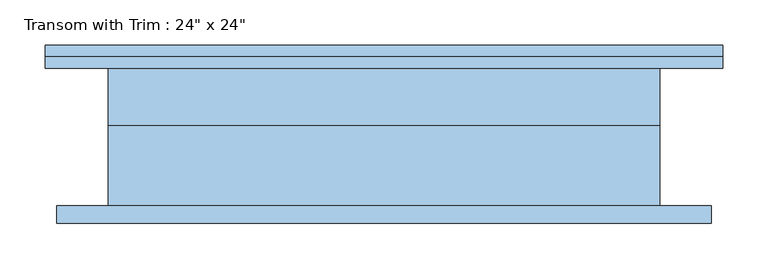
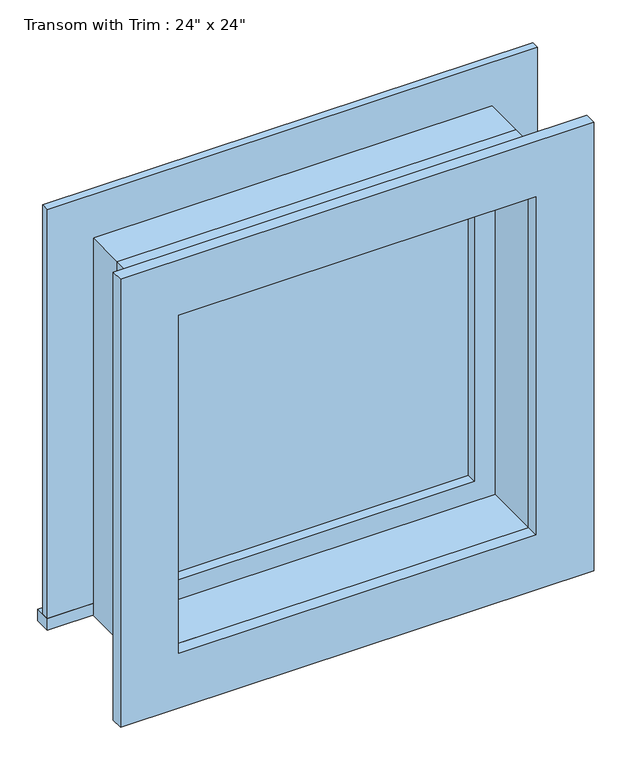
"""IFC4 building model written with IfcOpenShell, lengths in millimetres: window geometry."""

from ifc_helpers import new_model, si_unit, frame, origin, place, context, project, spatial, polyline, outline, extrude, source, transform, mapped, element, save


def window_3d781103(model_context):
    return source(origin(), model_context, "Body", "SweptSolid", [
        extrude(outline(polyline([(-412.75, 101.6), (336.55, 101.6), (336.55, 76.2), (-412.75, 76.2), (-412.75, 101.6)])), frame((0.0, 0.0, 2159.0), z_axis=(0.0, 0.0, 1.0), x_axis=(1.0, 0.0, 0.0)), (0.0, 0.0, 1.0), 19.05),
        extrude(outline(polyline([(2749.55, -323.85), (2749.55, 247.65), (2178.05, 247.65), (2178.05, 336.55), (2838.45, 336.55), (2838.45, -412.75), (2178.05, -412.75), (2178.05, -323.85), (2749.55, -323.85)])), frame((0.0, 76.2, 0.0), z_axis=(0.0, 1.0, 0.0), x_axis=(0.0, 0.0, 1.0)), (0.0, 0.0, 1.0), 12.7),
        extrude(outline(polyline([(2825.75, 323.85), (2825.75, -400.05), (2101.85, -400.05), (2101.85, 323.85), (2825.75, 323.85)]), holes=[polyline([(2736.85, 234.95), (2190.75, 234.95), (2190.75, -311.15), (2736.85, -311.15), (2736.85, 234.95)])]), frame((0.0, -95.25, 0.0), z_axis=(0.0, 1.0, 0.0), x_axis=(0.0, 0.0, 1.0)), (0.0, 0.0, 1.0), 19.05),
        extrude(outline(polyline([(203.2, 28.575), (-279.4, 28.575), (-279.4, 41.275), (203.2, 41.275), (203.2, 28.575)])), frame((0.0, 0.0, 2222.5), z_axis=(0.0, 0.0, 1.0), x_axis=(1.0, 0.0, 0.0)), (0.0, 0.0, 1.0), 482.6),
        extrude(outline(polyline([(2749.55, -323.85), (2178.05, -323.85), (2178.05, 247.65), (2749.55, 247.65), (2749.55, -323.85)]), holes=[polyline([(2705.1, -279.4), (2705.1, 203.2), (2222.5, 203.2), (2222.5, -279.4), (2705.1, -279.4)])]), frame((0.0, 12.7, 0.0), z_axis=(0.0, 1.0, 0.0), x_axis=(0.0, 0.0, 1.0)), (0.0, 0.0, 1.0), 44.45),
        extrude(outline(polyline([(2768.6, -342.9), (2159.0, -342.9), (2159.0, 266.7), (2768.6, 266.7), (2768.6, -342.9)]), holes=[polyline([(2736.85, -311.15), (2736.85, 234.95), (2190.75, 234.95), (2190.75, -311.15), (2736.85, -311.15)])]), frame((0.0, -76.2, 0.0), z_axis=(0.0, 1.0, 0.0), x_axis=(0.0, 0.0, 1.0)), (0.0, 0.0, 1.0), 88.9),
        extrude(outline(polyline([(2768.6, 266.7), (2768.6, -342.9), (2159.0, -342.9), (2159.0, 266.7), (2768.6, 266.7)]), holes=[polyline([(2749.55, 247.65), (2178.05, 247.65), (2178.05, -323.85), (2749.55, -323.85), (2749.55, 247.65)])]), frame((0.0, 12.7, 0.0), z_axis=(0.0, 1.0, 0.0), x_axis=(0.0, 0.0, 1.0)), (0.0, 0.0, 1.0), 63.5),
    ])


if __name__ == "__main__":
    model = new_model("IFC4")
    model_context = context("Model", 3, world=origin())
    ifc_project = project(units=[si_unit("LENGTHUNIT", "METRE", prefix="MILLI")], contexts=[model_context])
    site = spatial("IfcSite", under=ifc_project)
    building = spatial("IfcBuilding", under=site)
    placement = place(None, origin())
    window_shape = window_3d781103(model_context)
    element("IfcWindow", 1, ObjectType="Transom with Trim : 24\" x 24\"", at=placement, inside=building, context=model_context, shape_type="MappedRepresentation", body=[
        mapped(window_shape, transform((0.0, 0.0, 0.0), x_axis=(1.0, 0.0, 0.0), y_axis=(0.0, 1.0, 0.0), z_axis=(0.0, 0.0, 1.0))),
    ])
    save(model, "model.ifc")

# Revit data of these elements
# Type "Transom with Trim : 24\" x 24\""
#   Type Mark = "19"
#   Construction Type Id = "GSP4R"
#   Assembly Code = "B2020100"
#   Analytic Construction = "1/8 in Pilkington single glazing"
#   Visual Light Transmittance = 0.9
#   Solar Heat Gain Coefficient = 0.78
#   Heat Transfer Coefficient (U) = 0.6496 BTU/(h·ft²·°F)
#   Height = 2' - 0"
#   Default Sill Height = 7' - 1"
#   Trim Projection - Ext. = 0' - 0 1/2"
#   Trim Projection - Int. = 0' - 0 3/4"
#   Trim Width - Exterior = 0' - 3 1/2"
#   Trim Width - Interior = 0' - 3 1/2"
#   Width = 2' - 0"
#   Window Inset = 0' - 0 3/4"
#   Define Thermal Properties by = 1
#   Glass Pane Material = Glass
#   Sash Material = Sash
#   Trim Exterior Material = Trim
#   Trim Interior Material = Trim
#   Wall Closure = (empty or 0)
# Element 1 (IfcWindow, "Transom with Trim : 24\" x 24\"")
#   Materials on its faces: "Sash", "Trim", "Glass"
# Materials
#   "Glass": class "Glass", colour RGB 0 128 192, transparency 0.75, Description = "Soda Lime Glass", Cost = 0
#   "Sash": class "Wood", colour RGB 224 178 126, transparency 0
#   "Trim": class "Wood", colour RGB 224 178 126, transparency 0
